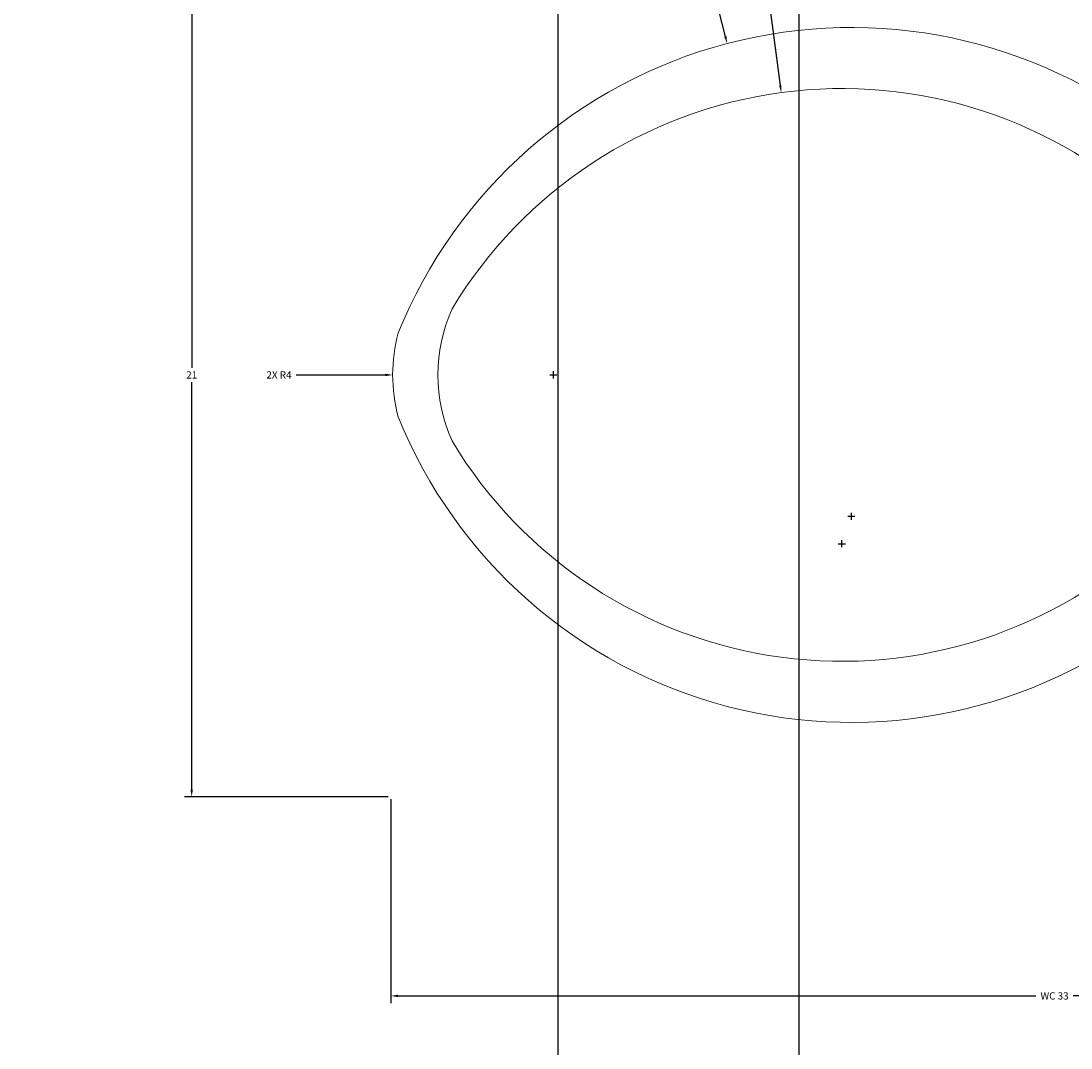
# Model space of a CAD drawing. Units: inches. Extents: x 2307 to 2544, y 2171 to 2540.
# Tile 46 of 52: x 2472 to 2498, y 2482 to 2507. Entities that reach past the tile are written whole.
import ezdxf

# ---------------------------------------------------------------- set-up
doc = ezdxf.new("R2010")
doc.units = ezdxf.units.IN
doc.layers.add('A-ANNO-DIMS', color=2, linetype='Continuous', lineweight=18)
doc.layers.add('A-FLOR-FIXT', color=9, linetype='Continuous', lineweight=18)
doc.styles.get("Standard").update_dxf_attribs({"font": 'arial.ttf'})
doc.dimstyles.get("Standard").update_dxf_attribs({"dimtxt": 0.18, "dimasz": 0.18, "dimexe": 0.18, "dimexo": 0.0625, "dimgap": 0.09, "dimtad": 0, "dimtih": 1, "dimtoh": 1, "dimdec": 4, "dimzin": 0, "dimdsep": 46, "dimtxsty": 'Standard', "dimcen": 0.09, "dimadec": 0, "dimazin": 0, "dimtfac": 1, "dimtdec": 4, "dimtofl": 0, "dimtmove": 0, "dimatfit": 3, "dimfxl": 1, "dimtolj": 1, "dimtzin": 0, "dimarcsym": 0})

# ---------------------------------------------------------------- blocks, each defined once
blk = doc.blocks.new('Toilet - top')
for centre, radius, start, end in [((3.52, -21.58), 12.169, 141.4691, 247.9714), ((4.2, -21.817), 11.329, 136.3677, 238.9468), ((-3.519, -21.58), 12.169, 292.0284, 38.5307), ((-4.2, -21.817), 11.329, 301.053, 43.6321), ((0, -27.876), 4, 245.7318, 294.2682), ((0, -29), 4, 254.8605, 285.1395)]:
    blk.add_arc(centre, radius, start, end)
blk = doc.blocks.new('*D20')
at = {"layer": 'A-ANNO-DIMS', "color": 0, "lineweight": -2, "transparency": 16777216}
for p, q in [((2481.532, 2488.115), (2481.532, 2483.04)), ((2514.578, 2488.115), (2514.578, 2483.04)), ((2481.712, 2483.22), (2497.588, 2483.22)), ((2514.398, 2483.22), (2498.522, 2483.22))]:
    blk.add_line(p, q, dxfattribs=at)
at = {"layer": 'A-ANNO-DIMS', "color": 0, "transparency": 16777216}
for points in [[(2481.712, 2483.25), (2481.712, 2483.19), (2481.532, 2483.22)], [(2514.398, 2483.25), (2514.398, 2483.19), (2514.578, 2483.22)]]:
    blk.add_solid(points, dxfattribs=at)
at = {"layer": 'Defpoints', "color": 0, "transparency": 16777216}
for p in [(2481.532, 2488.177), (2514.578, 2488.177), (2514.578, 2483.22)]:
    blk.add_point(p, dxfattribs=at)
at = {"layer": 'A-ANNO-DIMS', "color": 0, "transparency": 16777216, "insert": (2498.055, 2483.22), "char_height": 0.18, "attachment_point": 5}
blk.add_mtext('\\A1;WC 33', dxfattribs=at)
blk = doc.blocks.new('*D21')
at = {"layer": 'A-ANNO-DIMS', "color": 0, "lineweight": -2, "transparency": 16777216}
for p, q in [((2481.469, 2509.177), (2476.395, 2509.177)), ((2476.575, 2508.997), (2476.575, 2498.858)), ((2476.575, 2488.357), (2476.575, 2498.497)), ((2481.469, 2488.177), (2476.395, 2488.177))]:
    blk.add_line(p, q, dxfattribs=at)
at = {"layer": 'A-ANNO-DIMS', "color": 0, "transparency": 16777216}
for points in [[(2476.545, 2508.997), (2476.605, 2508.997), (2476.575, 2509.177)], [(2476.545, 2488.357), (2476.605, 2488.357), (2476.575, 2488.177)]]:
    blk.add_solid(points, dxfattribs=at)
at = {"layer": 'Defpoints', "color": 0, "transparency": 16777216}
for p in [(2481.532, 2509.177), (2476.575, 2488.177), (2481.532, 2488.177)]:
    blk.add_point(p, dxfattribs=at)
at = {"layer": 'A-ANNO-DIMS', "color": 0, "transparency": 16777216, "insert": (2476.575, 2498.677), "char_height": 0.18, "attachment_point": 5}
blk.add_mtext('\\A1;21', dxfattribs=at)
blk = doc.blocks.new('*D59')
at = {"layer": 'A-ANNO-DIMS', "color": 0, "lineweight": -2, "transparency": 16777216}
for p, q in [((2455.696, 2315.572), (2455.696, 2540.345)), ((2485.696, 2315.572), (2485.696, 2540.345)), ((2455.876, 2540.165), (2470.477, 2540.165)), ((2485.516, 2540.165), (2470.914, 2540.165))]:
    blk.add_line(p, q, dxfattribs=at)
at = {"layer": 'A-ANNO-DIMS', "color": 0, "transparency": 16777216}
for points in [[(2455.876, 2540.195), (2455.876, 2540.135), (2455.696, 2540.165)], [(2485.516, 2540.195), (2485.516, 2540.135), (2485.696, 2540.165)]]:
    blk.add_solid(points, dxfattribs=at)
at = {"layer": 'Defpoints', "color": 0, "transparency": 16777216}
for p in [(2455.696, 2540.165), (2455.696, 2315.51), (2485.696, 2315.51)]:
    blk.add_point(p, dxfattribs=at)
at = {"layer": 'A-ANNO-DIMS', "color": 0, "transparency": 16777216, "insert": (2470.696, 2540.165), "char_height": 0.18, "attachment_point": 5}
blk.add_mtext('\\A1;30', dxfattribs=at)
blk = doc.blocks.new('*D61')
at = {"layer": 'A-ANNO-DIMS', "color": 0, "lineweight": -2, "transparency": 16777216}
for p, q in [((2491.696, 2435.572), (2491.696, 2540.345)), ((2515.696, 2435.572), (2515.696, 2540.345)), ((2491.876, 2540.165), (2503.476, 2540.165)), ((2515.516, 2540.165), (2503.916, 2540.165))]:
    blk.add_line(p, q, dxfattribs=at)
at = {"layer": 'A-ANNO-DIMS', "color": 0, "transparency": 16777216}
for points in [[(2491.876, 2540.195), (2491.876, 2540.135), (2491.696, 2540.165)], [(2515.516, 2540.195), (2515.516, 2540.135), (2515.696, 2540.165)]]:
    blk.add_solid(points, dxfattribs=at)
at = {"layer": 'Defpoints', "color": 0, "transparency": 16777216}
for p in [(2515.696, 2540.165), (2491.696, 2435.51), (2515.696, 2435.51)]:
    blk.add_point(p, dxfattribs=at)
at = {"layer": 'A-ANNO-DIMS', "color": 0, "transparency": 16777216, "insert": (2503.696, 2540.165), "char_height": 0.18, "attachment_point": 5}
blk.add_mtext('\\A1;24', dxfattribs=at)
blk = doc.blocks.new('*D71')
at = {"layer": 'A-ANNO-DIMS', "color": 0, "lineweight": -2, "transparency": 16777216}
for p, q in [((2487.87, 2513.989), (2488.05, 2513.989)), ((2488.05, 2513.989), (2489.859, 2507.101)), ((2492.997, 2495.068), (2492.997, 2495.248)), ((2492.907, 2495.158), (2493.087, 2495.158))]:
    blk.add_line(p, q, dxfattribs=at)
at = {"layer": 'A-ANNO-DIMS', "color": 0, "transparency": 16777216}
blk.add_solid([(2489.888, 2507.109), (2489.83, 2507.094), (2489.905, 2506.927)], dxfattribs=at)
at = {"layer": 'Defpoints', "color": 0, "transparency": 16777216}
for p in [(2489.905, 2506.927), (2492.997, 2495.158)]:
    blk.add_point(p, dxfattribs=at)
at = {"layer": 'A-ANNO-DIMS', "color": 0, "transparency": 16777216, "insert": (2487.195, 2513.989), "char_height": 0.18, "attachment_point": 5}
blk.add_mtext('\\A1;2X R12.17', dxfattribs=at)
blk = doc.blocks.new('*D72')
at = {"layer": 'A-ANNO-DIMS', "color": 0, "lineweight": -2, "transparency": 16777216}
for p, q in [((2490.165, 2512.442), (2490.345, 2512.442)), ((2490.345, 2512.442), (2491.227, 2505.884)), ((2492.67, 2494.477), (2492.85, 2494.477)), ((2492.76, 2494.387), (2492.76, 2494.567))]:
    blk.add_line(p, q, dxfattribs=at)
at = {"layer": 'A-ANNO-DIMS', "color": 0, "transparency": 16777216}
blk.add_solid([(2491.257, 2505.888), (2491.197, 2505.88), (2491.251, 2505.705)], dxfattribs=at)
at = {"layer": 'Defpoints', "color": 0, "transparency": 16777216}
for p in [(2491.251, 2505.705), (2492.76, 2494.477)]:
    blk.add_point(p, dxfattribs=at)
at = {"layer": 'A-ANNO-DIMS', "color": 0, "transparency": 16777216, "insert": (2489.491, 2512.442), "char_height": 0.18, "attachment_point": 5}
blk.add_mtext('\\A1;2X R11.33', dxfattribs=at)
blk = doc.blocks.new('*D73')
at = {"layer": 'A-ANNO-DIMS', "color": 0, "lineweight": -2, "transparency": 16777216}
for p, q in [((2479.178, 2498.677), (2481.398, 2498.677)), ((2485.488, 2498.677), (2485.668, 2498.677)), ((2485.578, 2498.587), (2485.578, 2498.767))]:
    blk.add_line(p, q, dxfattribs=at)
at = {"layer": 'A-ANNO-DIMS', "color": 0, "transparency": 16777216}
blk.add_solid([(2481.398, 2498.707), (2481.398, 2498.647), (2481.578, 2498.677)], dxfattribs=at)
at = {"layer": 'Defpoints', "color": 0, "transparency": 16777216}
for p in [(2481.578, 2498.677), (2485.578, 2498.677)]:
    blk.add_point(p, dxfattribs=at)
at = {"layer": 'A-ANNO-DIMS', "color": 0, "transparency": 16777216, "insert": (2478.748, 2498.677), "char_height": 0.18, "attachment_point": 5}
blk.add_mtext('\\A1;2X R4', dxfattribs=at)

msp = doc.modelspace()

# ---------------------------------------------------------------- block references
at = {"layer": 'A-FLOR-FIXT', "rotation": 270}
msp.add_blockref('Toilet - top', (2514.5778, 2498.6772), dxfattribs=at)

# ---------------------------------------------------------------- dimensions: what is measured, and where the dimension line sits
at = {"layer": 'A-ANNO-DIMS'}
for base, p1, p2, picture, middle in [((2455.6958, 2540.1649), (2485.6958, 2315.5096), (2455.6958, 2315.5096), '*D59', (2470.6958, 2540.1649)), ((2515.6958, 2540.1649), (2491.6958, 2435.5096), (2515.6958, 2435.5096), '*D61', (2503.6958, 2540.1649))]:
    dim = msp.add_linear_dim(base=base, p1=p1, p2=p2, dimstyle='Standard', override={"dimdec": 0, "dimlfac": 1, "dimrnd": 0, "dimzin": 0, "dimdsep": 46, "dimlunit": 2}, dxfattribs=at)
    dim.commit()
    dim.dimension.update_dxf_attribs({"geometry": picture, "text_midpoint": middle})
for center, mpoint, override, picture, middle in [((2492.9973, 2495.1576), (2489.905, 2506.9272), {"dimdec": 2, "dimlfac": 1, "dimrnd": 0, "dimzin": 0, "dimdsep": 46, "dimlunit": 2}, '*D71', (2487.1948, 2513.9889)), ((2492.7604, 2494.4772), (2491.2509, 2505.7054), {"dimdec": 2, "dimlfac": 1, "dimrnd": 0, "dimzin": 0, "dimdsep": 46, "dimlunit": 2}, '*D72', (2489.4905, 2512.4423)), ((2485.5778, 2498.6771), (2481.5778, 2498.677), {"dimdec": 0, "dimlfac": 1, "dimrnd": 0, "dimzin": 0, "dimdsep": 46, "dimlunit": 2}, '*D73', (2479.1778, 2498.6769))]:
    dim = msp.add_radius_dim(center=center, mpoint=mpoint, text='2X <>', dimstyle='Standard', override=override, dxfattribs=at)
    dim.commit()
    dim.dimension.update_dxf_attribs({"geometry": picture, "text_midpoint": middle, "dimtype": 164})
dim = msp.add_linear_dim(base=(2476.5746, 2488.1772), p1=(2481.5315, 2509.1772), p2=(2481.5315, 2488.1772), angle=270, dimstyle='Standard', override={"dimdec": 0, "dimlfac": 1, "dimrnd": 0, "dimzin": 0, "dimdsep": 46, "dimlunit": 2}, dxfattribs=at)
dim.commit()
dim.dimension.update_dxf_attribs({"geometry": '*D21', "text_midpoint": (2476.5746, 2498.6772)})
dim = msp.add_linear_dim(base=(2514.5778, 2483.2202), p1=(2481.5315, 2488.1772), p2=(2514.5778, 2488.1772), text='WC <>', dimstyle='Standard', override={"dimdec": 0, "dimlfac": 1, "dimrnd": 0, "dimzin": 0, "dimdsep": 46, "dimlunit": 2}, dxfattribs=at)
dim.commit()
dim.dimension.update_dxf_attribs({"geometry": '*D20', "text_midpoint": (2498.0546, 2483.2202)})

doc.saveas('drawing.dxf')
